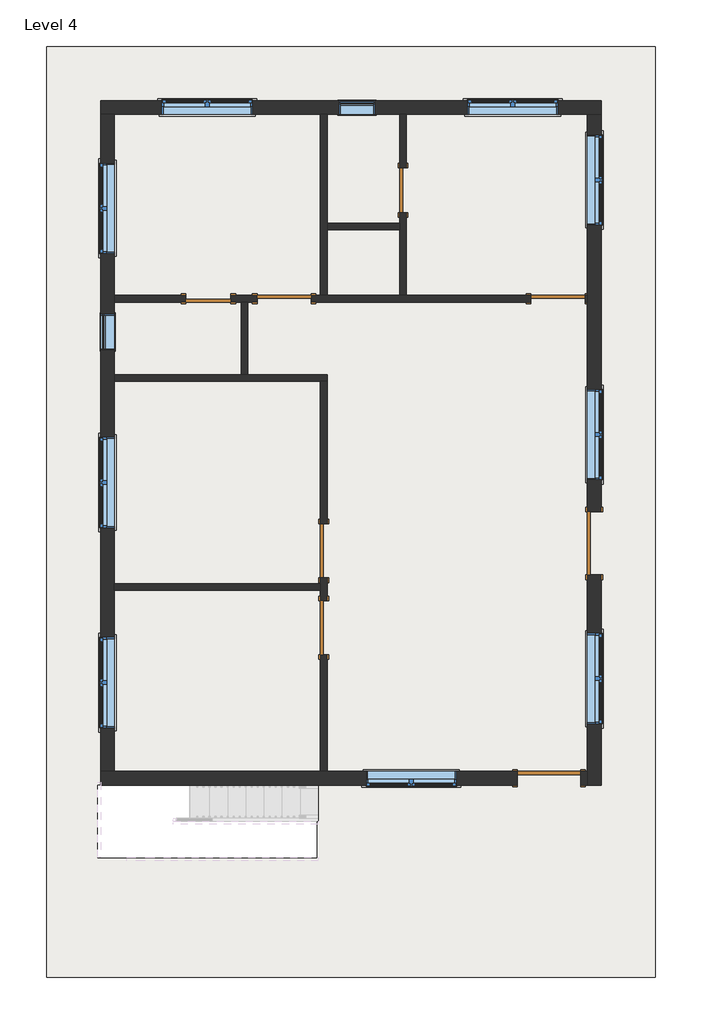
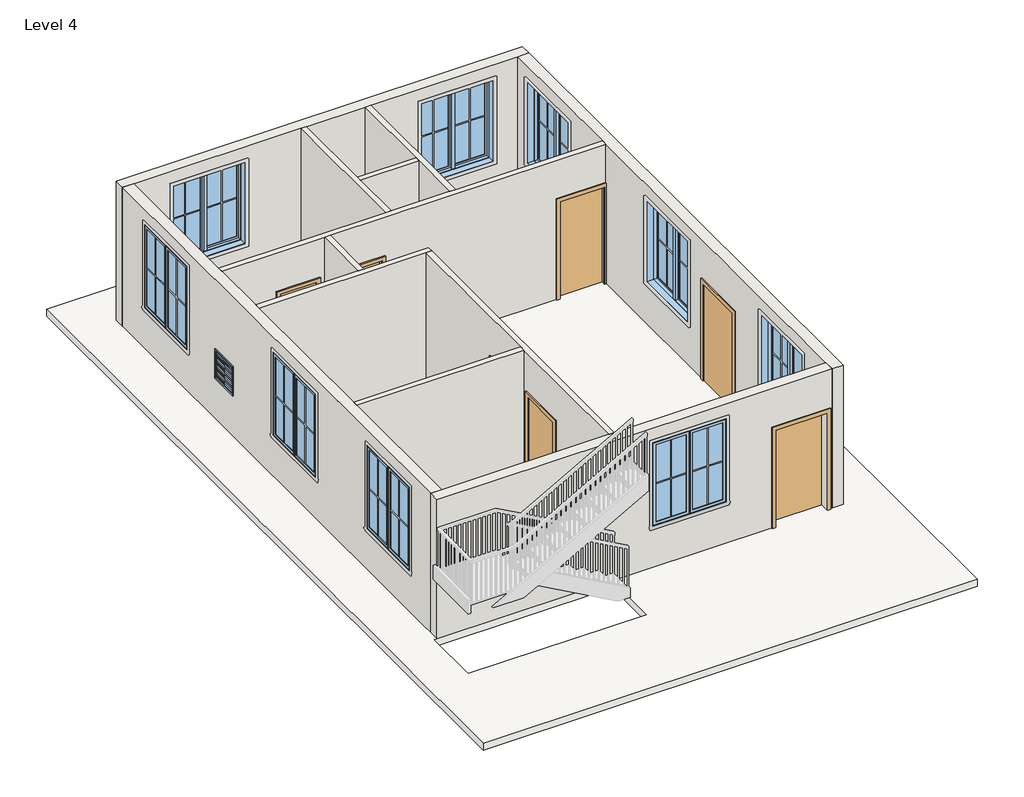
# One storey, part 1 of 3: 12 walls, 11 windows, 8 doors, 1 roof.
"""IFC4 building model written with IfcOpenShell, lengths in millimetres."""

from ifc_helpers import new_model, si_unit, frame, origin, place, context, project, spatial, polyline, outline, extrude, faceted_brep, transform, mapped, element, save
from components import door_78caadf7, single_flush_door_3_e5f9f3c4, single_flush_door_3_305aa2a5, door_9d399b00, door_0848dd25, window_casement_double_win_5_f93960c7, window_f2d8fef0

model = new_model("IFC4")

# Units and contexts
model_context = context("Model", 3, world=origin())
ifc_project = project(units=[si_unit("LENGTHUNIT", "METRE", prefix="MILLI")], contexts=[model_context])

# Site, building, storey
site = spatial("IfcSite", under=ifc_project)
building = spatial("IfcBuilding", under=site)
storey = spatial("IfcBuildingStorey", under=building, Name="Level 4", Elevation=6400.8)

# Doors
placement = place(None, origin())
door_shape = door_78caadf7(model_context)
element("IfcDoor", 1, ObjectType="Single-Flush : DOOR 2'6\"", at=placement, inside=storey, context=model_context, shape_type="MappedRepresentation", body=[
    mapped(door_shape, transform((-377.1698569, 4707.5566963, 6400.8), x_axis=(0.0, -1.0, 0.0), y_axis=(1.0, 0.0, 0.0), z_axis=(0.0, 0.0, 1.0))),
])
element("IfcDoor", 2, ObjectType="Single-Flush : DOOR 2'6\"", at=placement, inside=storey, context=model_context, shape_type="MappedRepresentation", body=[
    mapped(door_shape, transform((-3653.7698569, 2878.7566963, 6400.8), x_axis=(1.0, 0.0, 0.0), y_axis=(0.0, 1.0, 0.0), z_axis=(0.0, 0.0, 1.0))),
])
single_flush_door_3_shape = single_flush_door_3_e5f9f3c4(model_context)
element("IfcDoor", 3, ObjectType="Single-Flush : DOOR 3'", at=placement, inside=storey, context=model_context, shape_type="MappedRepresentation", body=[
    mapped(single_flush_door_3_shape, transform((-2377.4198569, 2878.7566963, 6400.8), x_axis=(1.0, 0.0, 0.0), y_axis=(0.0, 1.0, 0.0), z_axis=(0.0, 0.0, 1.0))),
])
element("IfcDoor", 4, ObjectType="Single-Flush : DOOR 3'", at=placement, inside=storey, context=model_context, shape_type="MappedRepresentation", body=[
    mapped(single_flush_door_3_shape, transform((2232.6801431, 2878.7566963, 6400.8), x_axis=(1.0, 0.0, 0.0), y_axis=(0.0, 1.0, 0.0), z_axis=(0.0, 0.0, 1.0))),
])
element("IfcDoor", 5, ObjectType="Single-Flush : DOOR 3'", at=placement, inside=storey, context=model_context, shape_type="MappedRepresentation", body=[
    mapped(single_flush_door_3_shape, transform((-1710.6698569, -2658.4433037, 6400.8), x_axis=(0.0, 1.0, 0.0), y_axis=(-1.0, 0.0, 0.0), z_axis=(0.0, 0.0, 1.0))),
])
single_flush_door_3_2_shape = single_flush_door_3_305aa2a5(model_context)
element("IfcDoor", 6, ObjectType="Single-Flush : DOOR 3'", at=placement, inside=storey, context=model_context, shape_type="MappedRepresentation", body=[
    mapped(single_flush_door_3_2_shape, transform((-1710.6698569, -1363.0433037, 6400.8), x_axis=(0.0, -1.0, 0.0), y_axis=(1.0, 0.0, 0.0), z_axis=(0.0, 0.0, 1.0))),
])
door_2_shape = door_9d399b00(model_context)
element("IfcDoor", 7, ObjectType="Single-Flush : DOOR 3'6\"", at=placement, inside=storey, context=model_context, shape_type="MappedRepresentation", body=[
    mapped(door_2_shape, transform((2080.2801431, -5192.0933037, 6400.8), x_axis=(1.0, 0.0, 0.0), y_axis=(0.0, 1.0, 0.0), z_axis=(0.0, 0.0, 1.0))),
])
door_3_shape = door_0848dd25(model_context)
element("IfcDoor", 8, ObjectType="Single-Flush : DOOR 3'6\"", at=placement, inside=storey, context=model_context, shape_type="MappedRepresentation", body=[
    mapped(door_3_shape, transform((2842.2801431, -1236.0433037, 6400.8), x_axis=(0.0, -1.0, 0.0), y_axis=(1.0, 0.0, 0.0), z_axis=(0.0, 0.0, 1.0))),
])

# Roof
element("IfcRoof", 9, ObjectType="ROOF 6\"", at=placement, inside=storey, context=model_context, shape_type="SweptSolid", body=[
    extrude(outline(polyline([(-6377.9198569, -8544.8933037), (-6377.9198569, 7126.9066963), (3870.9801431, 7126.9066963), (3870.9801431, -8544.8933037), (-6377.9198569, -8544.8933037)]), holes=[polyline([(-5514.3198569, -5306.3933037), (-5514.3198569, -6525.5933037), (-1831.3198569, -6525.5933037), (-1831.3198569, -5306.3933037), (-5514.3198569, -5306.3933037)])]), frame((0.0, 0.0, 6248.4), z_axis=(0.0, 0.0, 1.0), x_axis=(1.0, 0.0, 0.0)), (0.0, 0.0, 1.0), 152.4),
])

# Walls
element("IfcWall", 10, ObjectType="WALL 4.5\"", at=placement, inside=storey, context=model_context, shape_type="Brep", body=[
    faceted_brep([(2689.8801431, 2821.6066963, 8534.4), (2689.8801431, 2821.6066963, 6400.8), (2727.9801431, 2821.6066963, 6400.8), (2727.9801431, 2821.6066963, 9448.8), (-2987.0198569, 2821.6066963, 9448.8), (-3101.3198569, 2821.6066963, 9448.8), (-5234.9198569, 2821.6066963, 9448.8), (-5234.9198569, 2821.6066963, 6400.8), (-4034.7698569, 2821.6066963, 6400.8), (-4034.7698569, 2821.6066963, 8534.4), (-3272.7698569, 2821.6066963, 8534.4), (-3272.7698569, 2821.6066963, 6400.8), (-3101.3198569, 2821.6066963, 6400.8), (-2987.0198569, 2821.6066963, 6400.8), (-2834.6198569, 2821.6066963, 6400.8), (-2834.6198569, 2821.6066963, 8534.4), (-1920.2198569, 2821.6066963, 8534.4), (-1920.2198569, 2821.6066963, 6400.8), (1775.4801431, 2821.6066963, 6400.8), (1775.4801431, 2821.6066963, 8534.4), (2727.9801431, 2935.9066963, 6400.8), (2689.8801431, 2935.9066963, 6400.8), (2689.8801431, 2935.9066963, 8534.4), (1775.4801431, 2935.9066963, 8534.4), (1775.4801431, 2935.9066963, 6400.8), (-320.0198569, 2935.9066963, 6400.8), (-434.3198569, 2935.9066963, 6400.8), (-1653.5198569, 2935.9066963, 6400.8), (-1767.8198569, 2935.9066963, 6400.8), (-1920.2198569, 2935.9066963, 6400.8), (-1920.2198569, 2935.9066963, 8534.4), (-2834.6198569, 2935.9066963, 8534.4), (-2834.6198569, 2935.9066963, 6400.8), (-3272.7698569, 2935.9066963, 6400.8), (-3272.7698569, 2935.9066963, 8534.4), (-4034.7698569, 2935.9066963, 8534.4), (-4034.7698569, 2935.9066963, 6400.8), (-5234.9198569, 2935.9066963, 6400.8), (-5234.9198569, 2935.9066963, 9448.8), (-1767.8198569, 2935.9066963, 9448.8), (-1653.5198569, 2935.9066963, 9448.8), (-434.3198569, 2935.9066963, 9448.8), (-320.0198569, 2935.9066963, 9448.8), (2727.9801431, 2935.9066963, 9448.8)], [[[0, 1, 2, 3, 4, 5, 6, 7, 8, 9, 10, 11, 12, 13, 14, 15, 16, 17, 18, 19]], [[20, 21, 22, 23, 24, 25, 26, 27, 28, 29, 30, 31, 32, 33, 34, 35, 36, 37, 38, 39, 40, 41, 42, 43]], [[8, 7, 37, 36]], [[14, 13, 12, 11, 33, 32]], [[18, 17, 29, 28, 27, 26, 25, 24]], [[2, 1, 21, 20]], [[3, 2, 20, 43]], [[7, 6, 38, 37]], [[34, 33, 11, 10]], [[35, 34, 10, 9]], [[36, 35, 9, 8]], [[30, 29, 17, 16]], [[31, 30, 16, 15]], [[32, 31, 15, 14]], [[22, 21, 1, 0]], [[23, 22, 0, 19]], [[24, 23, 19, 18]], [[6, 5, 4, 3, 43, 42, 41, 40, 39, 38]]]),
])
element("IfcWall", 11, ObjectType="WALL 4.5\"", at=placement, inside=storey, context=model_context, shape_type="Brep", body=[
    faceted_brep([(-1767.8198569, 5983.9066963, 6400.8), (-1767.8198569, 2935.9066963, 6400.8), (-1767.8198569, 2935.9066963, 9448.8), (-1767.8198569, 5983.9066963, 9448.8), (-1653.5198569, 5983.9066963, 6400.8), (-1653.5198569, 5983.9066963, 9448.8), (-1653.5198569, 4155.1066963, 9448.8), (-1653.5198569, 4040.8066963, 9448.8), (-1653.5198569, 2935.9066963, 9448.8), (-1653.5198569, 2935.9066963, 6400.8), (-1653.5198569, 4040.8066963, 6400.8), (-1653.5198569, 4155.1066963, 6400.8)], [[[0, 1, 2, 3]], [[4, 5, 6, 7, 8, 9, 10, 11]], [[1, 0, 4, 11, 10, 9]], [[0, 3, 5, 4]], [[2, 1, 9, 8]], [[3, 2, 8, 7, 6, 5]]]),
])
element("IfcWall", 12, ObjectType="WALL 4.5\"", at=placement, inside=storey, context=model_context, shape_type="Brep", body=[
    faceted_brep([(-320.0198569, 2935.9066963, 6400.8), (-320.0198569, 4326.5566963, 6400.8), (-320.0198569, 4326.5566963, 8534.4), (-320.0198569, 5088.5566963, 8534.4), (-320.0198569, 5088.5566963, 6400.8), (-320.0198569, 5983.9066963, 6400.8), (-320.0198569, 5983.9066963, 9448.8), (-320.0198569, 2935.9066963, 9448.8), (-434.3198569, 4326.5566963, 8534.4), (-434.3198569, 4326.5566963, 6400.8), (-434.3198569, 4155.1066963, 6400.8), (-434.3198569, 4040.8066963, 6400.8), (-434.3198569, 2935.9066963, 6400.8), (-434.3198569, 2935.9066963, 9448.8), (-434.3198569, 4040.8066963, 9448.8), (-434.3198569, 4155.1066963, 9448.8), (-434.3198569, 5983.9066963, 9448.8), (-434.3198569, 5983.9066963, 6400.8), (-434.3198569, 5088.5566963, 6400.8), (-434.3198569, 5088.5566963, 8534.4)], [[[0, 1, 2, 3, 4, 5, 6, 7]], [[8, 9, 10, 11, 12, 13, 14, 15, 16, 17, 18, 19]], [[18, 17, 5, 4]], [[12, 11, 10, 9, 1, 0]], [[6, 5, 17, 16]], [[0, 7, 13, 12]], [[2, 1, 9, 8]], [[3, 2, 8, 19]], [[4, 3, 19, 18]], [[7, 6, 16, 15, 14, 13]]]),
])
element("IfcWall", 13, ObjectType="WALL 4.5\"", at=placement, inside=storey, context=model_context, shape_type="SweptSolid", body=[
    extrude(outline(polyline([(-434.3198569, 4040.8066963), (-1653.5198569, 4040.8066963), (-1653.5198569, 4155.1066963), (-434.3198569, 4155.1066963), (-434.3198569, 4040.8066963)])), frame((0.0, 0.0, 6400.8), z_axis=(0.0, 0.0, 1.0), x_axis=(1.0, 0.0, 0.0)), (0.0, 0.0, 1.0), 3048.0),
])
element("IfcWall", 14, ObjectType="WALL 4.5\"", at=placement, inside=storey, context=model_context, shape_type="Brep", body=[
    faceted_brep([(-5234.9198569, 1488.1066963, 6400.8), (-1767.8198569, 1488.1066963, 6400.8), (-1653.5198569, 1488.1066963, 6400.8), (-1653.5198569, 1488.1066963, 9448.8), (-1767.8198569, 1488.1066963, 9448.8), (-5234.9198569, 1488.1066963, 9448.8), (-5234.9198569, 1602.4066963, 6400.8), (-5234.9198569, 1602.4066963, 9448.8), (-3101.3198569, 1602.4066963, 9448.8), (-2987.0198569, 1602.4066963, 9448.8), (-1653.5198569, 1602.4066963, 9448.8), (-1653.5198569, 1602.4066963, 6400.8), (-2987.0198569, 1602.4066963, 6400.8), (-3101.3198569, 1602.4066963, 6400.8)], [[[0, 1, 2, 3, 4, 5]], [[6, 7, 8, 9, 10, 11, 12, 13]], [[2, 1, 0, 6, 13, 12, 11]], [[0, 5, 7, 6]], [[3, 2, 11, 10]], [[5, 4, 3, 10, 9, 8, 7]]]),
])
element("IfcWall", 15, ObjectType="WALL 4.5\"", at=placement, inside=storey, context=model_context, shape_type="Brep", body=[
    faceted_brep([(-1767.8198569, -1820.2433037, 6400.8), (-1767.8198569, -1915.4933037, 6400.8), (-1767.8198569, -2029.7933037, 6400.8), (-1767.8198569, -2201.2433037, 6400.8), (-1767.8198569, -2201.2433037, 8534.4), (-1767.8198569, -3115.6433037, 8534.4), (-1767.8198569, -3115.6433037, 6400.8), (-1767.8198569, -5077.7933037, 6400.8), (-1767.8198569, -5077.7933037, 9448.8), (-1767.8198569, -2029.7933037, 9448.8), (-1767.8198569, -1915.4933037, 9448.8), (-1767.8198569, 1488.1066963, 9448.8), (-1767.8198569, 1488.1066963, 6400.8), (-1767.8198569, -905.8433037, 6400.8), (-1767.8198569, -905.8433037, 8534.4), (-1767.8198569, -1820.2433037, 8534.4), (-1653.5198569, -2201.2433037, 8534.4), (-1653.5198569, -2201.2433037, 6400.8), (-1653.5198569, -1820.2433037, 6400.8), (-1653.5198569, -1820.2433037, 8534.4), (-1653.5198569, -905.8433037, 8534.4), (-1653.5198569, -905.8433037, 6400.8), (-1653.5198569, 1488.1066963, 6400.8), (-1653.5198569, 1488.1066963, 9448.8), (-1653.5198569, -5077.7933037, 9448.8), (-1653.5198569, -5077.7933037, 6400.8), (-1653.5198569, -3115.6433037, 6400.8), (-1653.5198569, -3115.6433037, 8534.4)], [[[0, 1, 2, 3, 4, 5, 6, 7, 8, 9, 10, 11, 12, 13, 14, 15]], [[16, 17, 18, 19, 20, 21, 22, 23, 24, 25, 26, 27]], [[13, 12, 22, 21]], [[26, 25, 7, 6]], [[18, 17, 3, 2, 1, 0]], [[12, 11, 23, 22]], [[8, 7, 25, 24]], [[19, 18, 0, 15]], [[20, 19, 15, 14]], [[21, 20, 14, 13]], [[4, 3, 17, 16]], [[5, 4, 16, 27]], [[6, 5, 27, 26]], [[11, 10, 9, 8, 24, 23]]]),
])
element("IfcWall", 16, ObjectType="WALL 4.5\"", at=placement, inside=storey, context=model_context, shape_type="SweptSolid", body=[
    extrude(outline(polyline([(-1767.8198569, -2029.7933037), (-5234.9198569, -2029.7933037), (-5234.9198569, -1915.4933037), (-1767.8198569, -1915.4933037), (-1767.8198569, -2029.7933037)])), frame((0.0, 0.0, 6400.8), z_axis=(0.0, 0.0, 1.0), x_axis=(1.0, 0.0, 0.0)), (0.0, 0.0, 1.0), 3048.0),
])
element("IfcWall", 17, ObjectType="WALL 4.5\"", at=placement, inside=storey, context=model_context, shape_type="SweptSolid", body=[
    extrude(outline(polyline([(-3101.3198569, 1602.4066963), (-3101.3198569, 2821.6066963), (-2987.0198569, 2821.6066963), (-2987.0198569, 1602.4066963), (-3101.3198569, 1602.4066963)])), frame((0.0, 0.0, 6400.8), z_axis=(0.0, 0.0, 1.0), x_axis=(1.0, 0.0, 0.0)), (0.0, 0.0, 1.0), 3048.0),
])
element("IfcWall", 18, ObjectType="WALL 9\"", at=placement, inside=storey, context=model_context, shape_type="Brep", body=[
    faceted_brep([(-5463.5198569, 5983.9066963, 6400.8), (-5234.9198569, 5983.9066963, 6400.8), (-1767.8198569, 5983.9066963, 6400.8), (-1653.5198569, 5983.9066963, 6400.8), (-434.3198569, 5983.9066963, 6400.8), (-320.0198569, 5983.9066963, 6400.8), (2727.9801431, 5983.9066963, 6400.8), (2956.5801431, 5983.9066963, 6400.8), (2956.5801431, 5983.9066963, 9448.8), (2727.9801431, 5983.9066963, 9448.8), (-320.0198569, 5983.9066963, 9448.8), (-434.3198569, 5983.9066963, 9448.8), (-1653.5198569, 5983.9066963, 9448.8), (-1767.8198569, 5983.9066963, 9448.8), (-5234.9198569, 5983.9066963, 9448.8), (-5463.5198569, 5983.9066963, 9448.8), (2232.6801431, 5983.9066963, 9144.0), (2232.6801431, 5983.9066963, 7315.2), (708.6801431, 5983.9066963, 7315.2), (708.6801431, 5983.9066963, 9144.0), (-2910.8198569, 5983.9066963, 9144.0), (-2910.8198569, 5983.9066963, 7315.2), (-4434.8198569, 5983.9066963, 7315.2), (-4434.8198569, 5983.9066963, 9144.0), (-1456.6698569, 5983.9066963, 7924.8), (-847.0698569, 5983.9066963, 7924.8), (-847.0698569, 5983.9066963, 7315.2), (-1456.6698569, 5983.9066963, 7315.2), (-5463.5198569, 6212.5066963, 6400.8), (-5463.5198569, 6212.5066963, 9448.8), (2956.5801431, 6212.5066963, 9448.8), (2956.5801431, 6212.5066963, 6400.8), (2232.6801431, 6212.5066963, 9144.0), (708.6801431, 6212.5066963, 9144.0), (708.6801431, 6212.5066963, 7315.2), (2232.6801431, 6212.5066963, 7315.2), (-2910.8198569, 6212.5066963, 9144.0), (-4434.8198569, 6212.5066963, 9144.0), (-4434.8198569, 6212.5066963, 7315.2), (-2910.8198569, 6212.5066963, 7315.2), (-1456.6698569, 6212.5066963, 7924.8), (-1456.6698569, 6212.5066963, 7315.2), (-847.0698569, 6212.5066963, 7315.2), (-847.0698569, 6212.5066963, 7924.8)], [[[0, 1, 2, 3, 4, 5, 6, 7, 8, 9, 10, 11, 12, 13, 14, 15], [16, 17, 18, 19], [20, 21, 22, 23], [24, 25, 26, 27]], [[28, 29, 30, 31], [32, 33, 34, 35], [36, 37, 38, 39], [40, 41, 42, 43]], [[7, 6, 5, 4, 3, 2, 1, 0, 28, 31]], [[8, 7, 31, 30]], [[0, 15, 29, 28]], [[17, 16, 32, 35]], [[18, 17, 35, 34]], [[19, 18, 34, 33]], [[16, 19, 33, 32]], [[21, 20, 36, 39]], [[22, 21, 39, 38]], [[23, 22, 38, 37]], [[20, 23, 37, 36]], [[41, 40, 24, 27]], [[42, 41, 27, 26]], [[43, 42, 26, 25]], [[40, 43, 25, 24]], [[15, 14, 13, 12, 11, 10, 9, 8, 30, 29]]]),
])
element("IfcWall", 19, ObjectType="WALL 9\"", at=placement, inside=storey, context=model_context, shape_type="Brep", body=[
    faceted_brep([(2727.9801431, -1769.4433037, 8534.4), (2727.9801431, -1769.4433037, 6400.8), (2727.9801431, -5077.7933037, 6400.8), (2727.9801431, -5306.3933037, 6400.8), (2727.9801431, -5306.3933037, 9448.8), (2727.9801431, -5077.7933037, 9448.8), (2727.9801431, 2821.6066963, 9448.8), (2727.9801431, 2935.9066963, 9448.8), (2727.9801431, 5983.9066963, 9448.8), (2727.9801431, 5983.9066963, 6400.8), (2727.9801431, 2935.9066963, 6400.8), (2727.9801431, 2821.6066963, 6400.8), (2727.9801431, -702.6433037, 6400.8), (2727.9801431, -702.6433037, 8534.4), (2727.9801431, 4117.0066963, 9144.0), (2727.9801431, 4117.0066963, 7315.2), (2727.9801431, 5641.0066963, 7315.2), (2727.9801431, 5641.0066963, 9144.0), (2727.9801431, -169.2433037, 9144.0), (2727.9801431, -169.2433037, 7315.2), (2727.9801431, 1354.7566963, 7315.2), (2727.9801431, 1354.7566963, 9144.0), (2727.9801431, -4277.6933037, 9144.0), (2727.9801431, -4277.6933037, 7315.2), (2727.9801431, -2753.6933037, 7315.2), (2727.9801431, -2753.6933037, 9144.0), (2956.5801431, -5306.3933037, 6400.8), (2956.5801431, -1769.4433037, 6400.8), (2956.5801431, -1769.4433037, 8534.4), (2956.5801431, -702.6433037, 8534.4), (2956.5801431, -702.6433037, 6400.8), (2956.5801431, 5983.9066963, 6400.8), (2956.5801431, 5983.9066963, 9448.8), (2956.5801431, -5306.3933037, 9448.8), (2956.5801431, 4117.0066963, 9144.0), (2956.5801431, 5641.0066963, 9144.0), (2956.5801431, 5641.0066963, 7315.2), (2956.5801431, 4117.0066963, 7315.2), (2956.5801431, -169.2433037, 9144.0), (2956.5801431, 1354.7566963, 9144.0), (2956.5801431, 1354.7566963, 7315.2), (2956.5801431, -169.2433037, 7315.2), (2956.5801431, -4277.6933037, 9144.0), (2956.5801431, -2753.6933037, 9144.0), (2956.5801431, -2753.6933037, 7315.2), (2956.5801431, -4277.6933037, 7315.2)], [[[0, 1, 2, 3, 4, 5, 6, 7, 8, 9, 10, 11, 12, 13], [14, 15, 16, 17], [18, 19, 20, 21], [22, 23, 24, 25]], [[26, 27, 28, 29, 30, 31, 32, 33], [34, 35, 36, 37], [38, 39, 40, 41], [42, 43, 44, 45]], [[3, 2, 1, 27, 26]], [[12, 11, 10, 9, 31, 30]], [[9, 8, 32, 31]], [[4, 3, 26, 33]], [[15, 14, 34, 37]], [[16, 15, 37, 36]], [[17, 16, 36, 35]], [[14, 17, 35, 34]], [[19, 18, 38, 41]], [[20, 19, 41, 40]], [[21, 20, 40, 39]], [[18, 21, 39, 38]], [[23, 22, 42, 45]], [[24, 23, 45, 44]], [[25, 24, 44, 43]], [[22, 25, 43, 42]], [[28, 27, 1, 0]], [[29, 28, 0, 13]], [[30, 29, 13, 12]], [[8, 7, 6, 5, 4, 33, 32]]]),
])
element("IfcWall", 20, ObjectType="WALL 9\"", at=placement, inside=storey, context=model_context, shape_type="Brep", body=[
    faceted_brep([(2727.9801431, -5077.7933037, 6400.8), (2613.6801431, -5077.7933037, 6400.8), (2613.6801431, -5077.7933037, 8534.4), (1546.8801431, -5077.7933037, 8534.4), (1546.8801431, -5077.7933037, 6400.8), (-1653.5198569, -5077.7933037, 6400.8), (-1767.8198569, -5077.7933037, 6400.8), (-5234.9198569, -5077.7933037, 6400.8), (-5463.5198569, -5077.7933037, 6400.8), (-5463.5198569, -5077.7933037, 9448.8), (-5234.9198569, -5077.7933037, 9448.8), (-1767.8198569, -5077.7933037, 9448.8), (-1653.5198569, -5077.7933037, 9448.8), (2727.9801431, -5077.7933037, 9448.8), (-999.4698569, -5077.7933037, 9144.0), (-999.4698569, -5077.7933037, 7315.2), (524.5301431, -5077.7933037, 7315.2), (524.5301431, -5077.7933037, 9144.0), (2613.6801431, -5306.3933037, 8534.4), (2613.6801431, -5306.3933037, 6400.8), (2727.9801431, -5306.3933037, 6400.8), (2727.9801431, -5306.3933037, 9448.8), (-1831.3198569, -5306.3933037, 9448.8), (-5463.5198569, -5306.3933037, 9448.8), (-5463.5198569, -5306.3933037, 6400.8), (1546.8801431, -5306.3933037, 6400.8), (1546.8801431, -5306.3933037, 8534.4), (-999.4698569, -5306.3933037, 9144.0), (524.5301431, -5306.3933037, 9144.0), (524.5301431, -5306.3933037, 7315.2), (-999.4698569, -5306.3933037, 7315.2)], [[[0, 1, 2, 3, 4, 5, 6, 7, 8, 9, 10, 11, 12, 13], [14, 15, 16, 17]], [[18, 19, 20, 21, 22, 23, 24, 25, 26], [27, 28, 29, 30]], [[25, 24, 8, 7, 6, 5, 4]], [[20, 19, 1, 0]], [[0, 13, 21, 20]], [[9, 8, 24, 23]], [[15, 14, 27, 30]], [[16, 15, 30, 29]], [[17, 16, 29, 28]], [[14, 17, 28, 27]], [[2, 1, 19, 18]], [[3, 2, 18, 26]], [[4, 3, 26, 25]], [[13, 12, 11, 10, 9, 23, 22, 21]]]),
])
element("IfcWall", 21, ObjectType="WALL 9\"", at=placement, inside=storey, context=model_context, shape_type="Brep", body=[
    faceted_brep([(-5234.9198569, -5077.7933037, 6400.8), (-5234.9198569, -2029.7933037, 6400.8), (-5234.9198569, -1915.4933037, 6400.8), (-5234.9198569, 1488.1066963, 6400.8), (-5234.9198569, 1602.4066963, 6400.8), (-5234.9198569, 2821.6066963, 6400.8), (-5234.9198569, 2935.9066963, 6400.8), (-5234.9198569, 5983.9066963, 6400.8), (-5234.9198569, 5983.9066963, 9448.8), (-5234.9198569, 2935.9066963, 9448.8), (-5234.9198569, 2821.6066963, 9448.8), (-5234.9198569, 1602.4066963, 9448.8), (-5234.9198569, 1488.1066963, 9448.8), (-5234.9198569, -1915.4933037, 9448.8), (-5234.9198569, -2029.7933037, 9448.8), (-5234.9198569, -5077.7933037, 9448.8), (-5234.9198569, -2820.3683037, 9144.0), (-5234.9198569, -2820.3683037, 7315.2), (-5234.9198569, -4344.3683037, 7315.2), (-5234.9198569, -4344.3683037, 9144.0), (-5234.9198569, 548.3066963, 9144.0), (-5234.9198569, 548.3066963, 7315.2), (-5234.9198569, -975.6933037, 7315.2), (-5234.9198569, -975.6933037, 9144.0), (-5234.9198569, 5164.7566963, 9144.0), (-5234.9198569, 5164.7566963, 7315.2), (-5234.9198569, 3640.7566963, 7315.2), (-5234.9198569, 3640.7566963, 9144.0), (-5234.9198569, 2015.1566963, 7924.8), (-5234.9198569, 2624.7566963, 7924.8), (-5234.9198569, 2624.7566963, 7315.2), (-5234.9198569, 2015.1566963, 7315.2), (-5463.5198569, -5077.7933037, 6400.8), (-5463.5198569, -5077.7933037, 9448.8), (-5463.5198569, 5983.9066963, 9448.8), (-5463.5198569, 5983.9066963, 6400.8), (-5463.5198569, -2820.3683037, 9144.0), (-5463.5198569, -4344.3683037, 9144.0), (-5463.5198569, -4344.3683037, 7315.2), (-5463.5198569, -2820.3683037, 7315.2), (-5463.5198569, 548.3066963, 9144.0), (-5463.5198569, -975.6933037, 9144.0), (-5463.5198569, -975.6933037, 7315.2), (-5463.5198569, 548.3066963, 7315.2), (-5463.5198569, 5164.7566963, 9144.0), (-5463.5198569, 3640.7566963, 9144.0), (-5463.5198569, 3640.7566963, 7315.2), (-5463.5198569, 5164.7566963, 7315.2), (-5463.5198569, 2015.1566963, 7924.8), (-5463.5198569, 2015.1566963, 7315.2), (-5463.5198569, 2624.7566963, 7315.2), (-5463.5198569, 2624.7566963, 7924.8)], [[[0, 1, 2, 3, 4, 5, 6, 7, 8, 9, 10, 11, 12, 13, 14, 15], [16, 17, 18, 19], [20, 21, 22, 23], [24, 25, 26, 27], [28, 29, 30, 31]], [[32, 33, 34, 35], [36, 37, 38, 39], [40, 41, 42, 43], [44, 45, 46, 47], [48, 49, 50, 51]], [[7, 6, 5, 4, 3, 2, 1, 0, 32, 35]], [[8, 7, 35, 34]], [[0, 15, 33, 32]], [[17, 16, 36, 39]], [[18, 17, 39, 38]], [[19, 18, 38, 37]], [[16, 19, 37, 36]], [[21, 20, 40, 43]], [[22, 21, 43, 42]], [[23, 22, 42, 41]], [[20, 23, 41, 40]], [[25, 24, 44, 47]], [[26, 25, 47, 46]], [[27, 26, 46, 45]], [[24, 27, 45, 44]], [[49, 48, 28, 31]], [[50, 49, 31, 30]], [[51, 50, 30, 29]], [[48, 51, 29, 28]], [[15, 14, 13, 12, 11, 10, 9, 8, 34, 33]]]),
])

# Windows
window_casement_double_win_5_shape = window_casement_double_win_5_f93960c7(model_context)
element("IfcWindow", 22, ObjectType="Window-Casement-Double : WIN 5'", at=placement, inside=storey, context=model_context, shape_type="MappedRepresentation", body=[
    mapped(window_casement_double_win_5_shape, transform((-5349.2198569, -3582.3683037, 6400.8), x_axis=(0.0, 1.0, 0.0), y_axis=(-1.0, 0.0, 0.0), z_axis=(0.0, 0.0, 1.0))),
])
element("IfcWindow", 23, ObjectType="Window-Casement-Double : WIN 5'", at=placement, inside=storey, context=model_context, shape_type="MappedRepresentation", body=[
    mapped(window_casement_double_win_5_shape, transform((-5349.2198569, -213.6933037, 6400.8), x_axis=(0.0, 1.0, 0.0), y_axis=(-1.0, 0.0, 0.0), z_axis=(0.0, 0.0, 1.0))),
])
element("IfcWindow", 24, ObjectType="Window-Casement-Double : WIN 5'", at=placement, inside=storey, context=model_context, shape_type="MappedRepresentation", body=[
    mapped(window_casement_double_win_5_shape, transform((-5349.2198569, 4402.7566963, 6400.8), x_axis=(0.0, 1.0, 0.0), y_axis=(-1.0, 0.0, 0.0), z_axis=(0.0, 0.0, 1.0))),
])
element("IfcWindow", 25, ObjectType="Window-Casement-Double : WIN 5'", at=placement, inside=storey, context=model_context, shape_type="MappedRepresentation", body=[
    mapped(window_casement_double_win_5_shape, transform((2842.2801431, 4879.0066963, 6400.8), x_axis=(0.0, -1.0, 0.0), y_axis=(1.0, 0.0, 0.0), z_axis=(0.0, 0.0, 1.0))),
])
element("IfcWindow", 26, ObjectType="Window-Casement-Double : WIN 5'", at=placement, inside=storey, context=model_context, shape_type="MappedRepresentation", body=[
    mapped(window_casement_double_win_5_shape, transform((2842.2801431, 592.7566963, 6400.8), x_axis=(0.0, -1.0, 0.0), y_axis=(1.0, 0.0, 0.0), z_axis=(0.0, 0.0, 1.0))),
])
element("IfcWindow", 27, ObjectType="Window-Casement-Double : WIN 5'", at=placement, inside=storey, context=model_context, shape_type="MappedRepresentation", body=[
    mapped(window_casement_double_win_5_shape, transform((2842.2801431, -3515.6933037, 6400.8), x_axis=(0.0, -1.0, 0.0), y_axis=(1.0, 0.0, 0.0), z_axis=(0.0, 0.0, 1.0))),
])
element("IfcWindow", 28, ObjectType="Window-Casement-Double : WIN 5'", at=placement, inside=storey, context=model_context, shape_type="MappedRepresentation", body=[
    mapped(window_casement_double_win_5_shape, transform((-237.4698569, -5192.0933037, 6400.8), x_axis=(-1.0, 0.0, 0.0), y_axis=(0.0, -1.0, 0.0), z_axis=(0.0, 0.0, 1.0))),
])
element("IfcWindow", 29, ObjectType="Window-Casement-Double : WIN 5'", at=placement, inside=storey, context=model_context, shape_type="MappedRepresentation", body=[
    mapped(window_casement_double_win_5_shape, transform((1470.6801431, 6098.2066963, 6400.8), x_axis=(1.0, 0.0, 0.0), y_axis=(0.0, 1.0, 0.0), z_axis=(0.0, 0.0, 1.0))),
])
element("IfcWindow", 30, ObjectType="Window-Casement-Double : WIN 5'", at=placement, inside=storey, context=model_context, shape_type="MappedRepresentation", body=[
    mapped(window_casement_double_win_5_shape, transform((-3672.8198569, 6098.2066963, 6400.8), x_axis=(1.0, 0.0, 0.0), y_axis=(0.0, 1.0, 0.0), z_axis=(0.0, 0.0, 1.0))),
])
window_shape = window_f2d8fef0(model_context)
element("IfcWindow", 31, ObjectType="Window-Louvers : 24\" x 24\"", at=placement, inside=storey, context=model_context, shape_type="MappedRepresentation", body=[
    mapped(window_shape, transform((-1151.8698569, 6104.5566963, 6400.8), x_axis=(1.0, 0.0, 0.0), y_axis=(0.0, 1.0, 0.0), z_axis=(0.0, 0.0, 1.0))),
])
element("IfcWindow", 32, ObjectType="Window-Louvers : 24\" x 24\"", at=placement, inside=storey, context=model_context, shape_type="MappedRepresentation", body=[
    mapped(window_shape, transform((-5355.5698569, 2319.9566963, 6400.8), x_axis=(0.0, 1.0, 0.0), y_axis=(-1.0, 0.0, 0.0), z_axis=(0.0, 0.0, 1.0))),
])

save(model, "model.ifc")

# Revit data of these elements
# Type "Single-Flush : DOOR 2'6\""
#   Type Mark = "10"
#   Construction Type Id = "MDOOR"
#   Assembly Code = "C1020"
#   Analytic Construction = "Metal"
#   Thickness = 0' - 2"
#   Heat Transfer Coefficient (U) = 0.651978 BTU/(h·ft²·°F)
#   Height = 7' - 0"
#   Trim Projection Ext = 0' - 1"
#   Trim Projection Int = 0' - 1"
#   Trim Width = 0' - 3"
#   Width = 2' - 6"
#   Define Thermal Properties by = 1
#   Door Material = Door - Panel
#   Frame Material = Door - Frame
#   Visual Light Transmittance = 0
#   Solar Heat Gain Coefficient = 0
#   Function = (empty or 0)
#   Wall Closure = (empty or 0)
# Type "Single-Flush : DOOR 3'"
#   Type Mark = "8"
#   Construction Type Id = "MDOOR"
#   Assembly Code = "C1020"
#   Analytic Construction = "Metal"
#   Thickness = 0' - 2"
#   Heat Transfer Coefficient (U) = 0.651978 BTU/(h·ft²·°F)
#   Height = 7' - 0"
#   Trim Projection Ext = 0' - 1"
#   Trim Projection Int = 0' - 1"
#   Trim Width = 0' - 3"
#   Width = 3' - 0"
#   Define Thermal Properties by = 1
#   Door Material = Door - Panel
#   Frame Material = Door - Frame
#   Visual Light Transmittance = 0
#   Solar Heat Gain Coefficient = 0
#   Function = (empty or 0)
#   Wall Closure = (empty or 0)
# Type "Single-Flush : DOOR 3'6\""
#   Type Mark = "9"
#   Construction Type Id = "MDOOR"
#   Assembly Code = "C1020"
#   Analytic Construction = "Metal"
#   Thickness = 0' - 2"
#   Heat Transfer Coefficient (U) = 0.651978 BTU/(h·ft²·°F)
#   Height = 7' - 0"
#   Trim Projection Ext = 0' - 1"
#   Trim Projection Int = 0' - 1"
#   Trim Width = 0' - 3"
#   Width = 3' - 6"
#   Define Thermal Properties by = 1
#   Door Material = Door - Panel
#   Frame Material = Door - Frame
#   Visual Light Transmittance = 0
#   Solar Heat Gain Coefficient = 0
#   Function = (empty or 0)
#   Wall Closure = (empty or 0)
# Type "ROOF 6\""
#   Assembly Code = "B1020"
#   Layers, outside or top first: 0' - 6" no material (function 1)
# Type "WALL 4.5\""
#   Assembly Code = "B2010"
#   Layers, outside or top first: 0' - 4 1/2" no material (function 1)
# Type "WALL 9\""
#   Assembly Code = "B2010"
#   Layers, outside or top first: 0' - 9" no material (function 1)
# Type "Window-Casement-Double : WIN 5'"
#   Type Mark = "20"
#   Fire Rating = "0.5h"
#   Assembly Code = "B2020100"
#   Analytic Construction = "Double glazing - domestic"
#   Frame Extension [instance default] = 0' - 0 1/4"
#   Window Inset [instance default] = 0' - 0"
#   Wall Thickness [instance default] = 0' - 6"
#   Interior Wall Closure [instance default] = 0' - 2 1/4"
#   Half Width = 2' - 6"
#   Visual Light Transmittance = 0.81
#   Thermal Resistance (R) = 1.8146 (h·ft²·°F)/BTU
#   Solar Heat Gain Coefficient = 0.76
#   Rough Width = 5' - 0 1/2"
#   Rough Height = 6' - 0 1/2"
#   Height = 6' - 0"
#   Heat Transfer Coefficient (U) = 0.5511 BTU/(h·ft²·°F)
#   Exterior Wall Closure [instance default] = 0' - 1 1/4"
#   Extension Jamb [instance default] = 0' - 2 1/4"
#   Default Sill Height = 3' - 0"
#   Width = 5' - 0"
#   Muntin Visibility = yes
#   Interior Trim Visibility [instance default] = yes
#   Exterior Trim Visibility [instance default] = yes
#   Extension Jamb Visibility [instance default] = yes
#   Interior Trim Material = Wood - Stained
#   Muntin Pattern = Muntin Pattern_2x2 : Muntin Pattern_2x2
#   Interior Trim = Trim-Window-Interior-Flat : Picture Frame
#   Interior Frame Material = Wood - Stained
#   Glass Panel Material = Glass
#   Exterior Trim Material = Clad - White
#   Exterior Trim = Trim-Window-Exterior-Flat : with Sill
#   Exterior Frame Material = Clad - White
#   Wall Closure = (empty or 0)
# Type "Window-Louvers : 24\" x 24\""
#   Type Mark = "21"
#   Construction Type Id = "GSP4R"
#   Assembly Code = "B20"
#   Analytic Construction = "1/8 in Pilkington single glazing"
#   Visual Light Transmittance = 0.9
#   Thermal Resistance (R) = 1.53941 (h·ft²·°F)/BTU
#   Solar Heat Gain Coefficient = 0.78
#   Max Height = 1' - 11.74264"
#   Height = 2' - 0"
#   Heat Transfer Coefficient (U) = 0.6496 BTU/(h·ft²·°F)
#   Blade Width [instance default] = 1' - 10 1/2"
#   Blade Vertical Thickness = 0' - 0.35355"
#   Blade Thickness = 0' - 0 1/4"
#   Blade Spacing = 0' - 1 1/2"
#   Blade Height = 0' - 1.85355"
#   Blade Depth = 0' - 3"
#   Blade Angle = 45.00°
#   Default Sill Height = 3' - 0"
#   Trim Projection_Exterior = 0' - 0 1/2"
#   Trim Projection_Interior = 0' - 0 1/2"
#   Trim Width_Exterior = 0' - 1 1/2"
#   Trim Width_Interior = 0' - 1 1/2"
#   Width = 2' - 0"
#   Max Blade Count = 12
#   Define Thermal Properties by = 1
#   Blade Count = 12
#   Frame Material = Birch
#   Louver Material = Birch
#   Trim Exterior Material = Birch
#   Trim Interior Material = Birch
#   Wall Closure = (empty or 0)
# Elements 1, 2 (IfcDoor, "Single-Flush : DOOR 2'6\"")
#   Phase Created = New Construction
#   Materials on its faces: "Door - Frame", "Door - Panel"
# Elements 3, 4, 5, 6 (IfcDoor, "Single-Flush : DOOR 3'")
#   Phase Created = New Construction
#   Materials on its faces: "Door - Frame", "Door - Panel"
# Elements 7, 8 (IfcDoor, "Single-Flush : DOOR 3'6\"")
#   Phase Created = New Construction
#   Materials on its faces: "Door - Frame", "Door - Panel"
# Element 9 (IfcRoof, "ROOF 6\"")
#   built-in parameter 1001705 = 21 (stored number, unit not read)
#   built-in parameter 1001701 = -0.5 (stored number, unit not read)
#   built-in parameter 1001710 = 33615
#   Phase Created = New Construction
#   Materials on its faces: "Default Roof", "Parking Stripe", "Wood - Stained"
# Elements 10, 11, 12, 13, 14, 15, 16, 17 (IfcWall, "WALL 4.5\"")
#   Top Offset = 0' - 0"
#   Base Offset = 0' - 0"
#   Unconnected Height = 10' - 0"
#   wall height = 10' - 0"
#   Phase Created = New Construction
#   Base Constraint = Level 4
#   Materials on its faces: "Default Wall"
# Elements 18, 19, 20, 21 (IfcWall, "WALL 9\"")
#   Top Offset = 0' - 0"
#   Base Offset = 0' - 0"
#   Unconnected Height = 10' - 0"
#   wall height = 10' - 0"
#   Phase Created = New Construction
#   Base Constraint = Level 4
#   Materials on its faces: "Default Wall", "Cherry"
# Element 22 (IfcWindow, "Window-Casement-Double : WIN 5'")
#   Mark = "23"
#   Window Inset = 0' - 0"
#   Interior Wall Closure = 0' - 2 1/4"
#   Frame Extension = 0' - 0 1/4"
#   Exterior Wall Closure = 0' - 1 1/4"
#   Interior Trim Visibility = yes
#   Exterior Trim Visibility = yes
#   Phase Created = New Construction
#   Materials on its faces: "Wood - Stained", "Glass", "Clad - White"
# Element 23 (IfcWindow, "Window-Casement-Double : WIN 5'")
#   Mark = "24"
#   Window Inset = 0' - 0"
#   Interior Wall Closure = 0' - 2 1/4"
#   Frame Extension = 0' - 0 1/4"
#   Exterior Wall Closure = 0' - 1 1/4"
#   Interior Trim Visibility = yes
#   Exterior Trim Visibility = yes
#   Phase Created = New Construction
#   Materials on its faces: "Wood - Stained", "Glass", "Clad - White"
# Element 24 (IfcWindow, "Window-Casement-Double : WIN 5'")
#   Mark = "25"
#   Window Inset = 0' - 0"
#   Interior Wall Closure = 0' - 2 1/4"
#   Frame Extension = 0' - 0 1/4"
#   Exterior Wall Closure = 0' - 1 1/4"
#   Interior Trim Visibility = yes
#   Exterior Trim Visibility = yes
#   Phase Created = New Construction
#   Materials on its faces: "Wood - Stained", "Glass", "Clad - White"
# Element 25 (IfcWindow, "Window-Casement-Double : WIN 5'")
#   Mark = "26"
#   Window Inset = 0' - 0"
#   Interior Wall Closure = 0' - 2 1/4"
#   Frame Extension = 0' - 0 1/4"
#   Exterior Wall Closure = 0' - 1 1/4"
#   Interior Trim Visibility = yes
#   Exterior Trim Visibility = yes
#   Phase Created = New Construction
#   Materials on its faces: "Wood - Stained", "Glass", "Clad - White"
# Element 26 (IfcWindow, "Window-Casement-Double : WIN 5'")
#   Mark = "27"
#   Window Inset = 0' - 0"
#   Interior Wall Closure = 0' - 2 1/4"
#   Frame Extension = 0' - 0 1/4"
#   Exterior Wall Closure = 0' - 1 1/4"
#   Interior Trim Visibility = yes
#   Exterior Trim Visibility = yes
#   Phase Created = New Construction
#   Materials on its faces: "Wood - Stained", "Glass", "Clad - White"
# Element 27 (IfcWindow, "Window-Casement-Double : WIN 5'")
#   Mark = "28"
#   Window Inset = 0' - 0"
#   Interior Wall Closure = 0' - 2 1/4"
#   Frame Extension = 0' - 0 1/4"
#   Exterior Wall Closure = 0' - 1 1/4"
#   Interior Trim Visibility = yes
#   Exterior Trim Visibility = yes
#   Phase Created = New Construction
#   Materials on its faces: "Wood - Stained", "Glass", "Clad - White"
# Element 28 (IfcWindow, "Window-Casement-Double : WIN 5'")
#   Mark = "29"
#   Window Inset = 0' - 0"
#   Interior Wall Closure = 0' - 2 1/4"
#   Frame Extension = 0' - 0 1/4"
#   Exterior Wall Closure = 0' - 1 1/4"
#   Interior Trim Visibility = yes
#   Exterior Trim Visibility = yes
#   Phase Created = New Construction
#   Materials on its faces: "Wood - Stained", "Glass", "Clad - White"
# Element 29 (IfcWindow, "Window-Casement-Double : WIN 5'")
#   Mark = "30"
#   Window Inset = 0' - 0"
#   Interior Wall Closure = 0' - 2 1/4"
#   Frame Extension = 0' - 0 1/4"
#   Exterior Wall Closure = 0' - 1 1/4"
#   Interior Trim Visibility = yes
#   Exterior Trim Visibility = yes
#   Phase Created = New Construction
#   Materials on its faces: "Wood - Stained", "Glass", "Clad - White"
# Element 30 (IfcWindow, "Window-Casement-Double : WIN 5'")
#   Mark = "31"
#   Window Inset = 0' - 0"
#   Interior Wall Closure = 0' - 2 1/4"
#   Frame Extension = 0' - 0 1/4"
#   Exterior Wall Closure = 0' - 1 1/4"
#   Interior Trim Visibility = yes
#   Exterior Trim Visibility = yes
#   Phase Created = New Construction
#   Materials on its faces: "Wood - Stained", "Glass", "Clad - White"
# Element 31 (IfcWindow, "Window-Louvers : 24\" x 24\"")
#   Mark = "32"
#   Blade Width = 1' - 10 1/2"
#   Phase Created = New Construction
#   Materials on its faces: "Birch"
# Element 32 (IfcWindow, "Window-Louvers : 24\" x 24\"")
#   Mark = "33"
#   Blade Width = 1' - 10 1/2"
#   Phase Created = New Construction
#   Materials on its faces: "Birch"
# Materials
#   "Door - Panel": class "Wood", colour RGB 210 159 95, transparency 0, Cost = 0
#   "Door - Frame": colour RGB 118 70 51, transparency 0, Cost = 0
#   "Wood - Stained": class "Wood", colour RGB 224 178 126, transparency 0, Cost = 0
#   "Glass": class "Glass", colour RGB 0 128 192, transparency 0.75, Description = "Soda Lime Glass", Cost = 0
#   "Clad - White": class "Wood", colour RGB 242 242 238, transparency 0, Cost = 0
#   "Birch": class "Wood", colour RGB 224 178 126, transparency 0, Description = "Betula Alleghaniensis", Cost = 0
#   "Default Roof": colour RGB 88 101 114, transparency 0, Cost = 0
#   "Parking Stripe": class "Paint", colour RGB 250 250 91, transparency 0, Cost = 0
#   "Default Wall": colour RGB 128 128 128, transparency 0, Cost = 0
#   "Cherry": class "Wood", colour RGB 226 177 128, transparency 0, Description = "Prunus Serotina", Cost = 0
